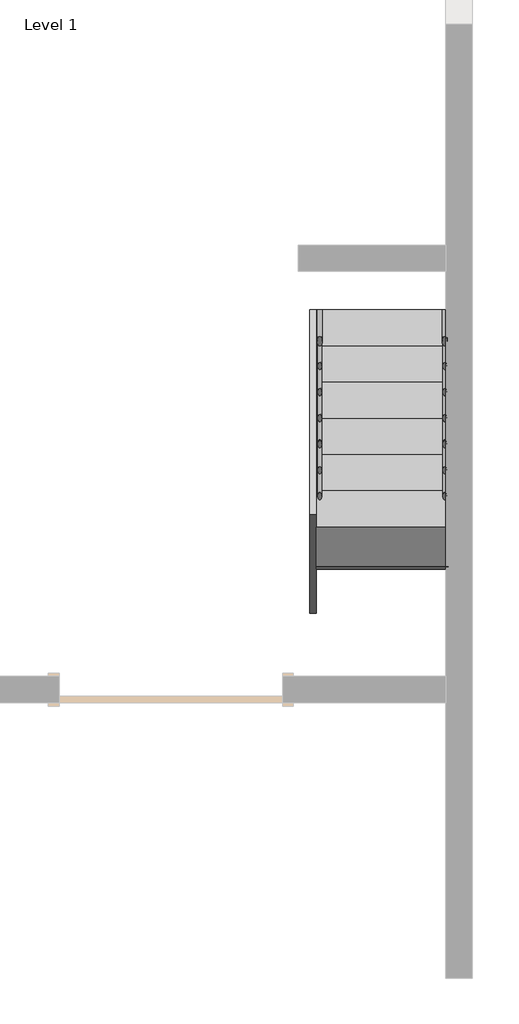
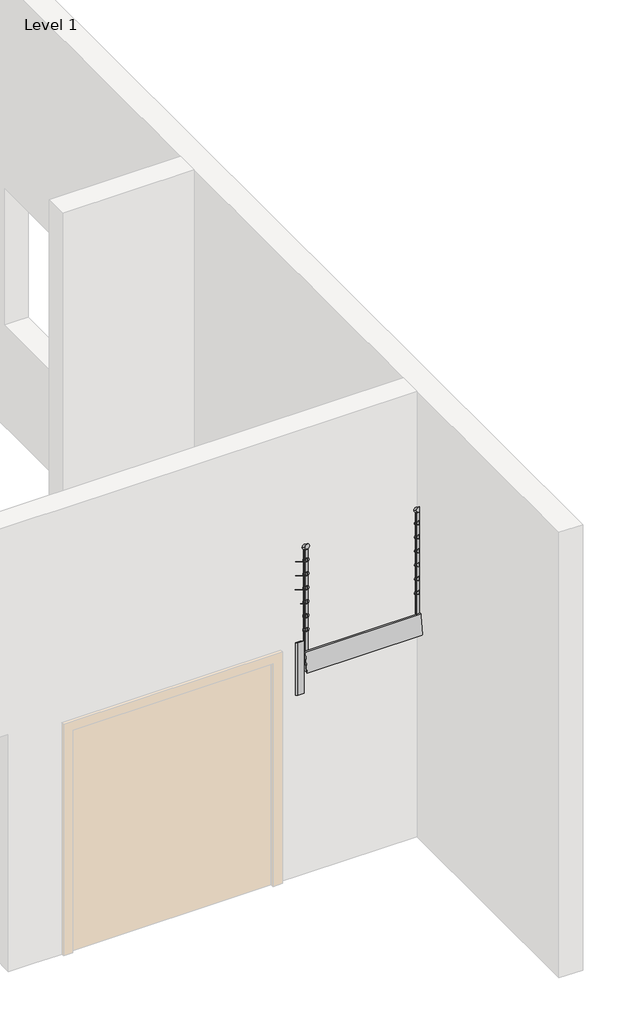
# One storey, part 2 of 2: 2 members, 2 railings, 1 stair flight.
"""IFC4 building model written with IfcOpenShell, lengths in millimetres."""

from ifc_helpers import new_model, si_unit, frame, origin, place, context, project, spatial, polyline, circle_curve, ellipse_curve, outline, extrude, transform, mapped, element, save
from ifc_brep_helpers import plane_surface, cylinder_surface, advanced_brep
from components import stair_flight_50mm_tread_25mm_nosing_13mm_riser_4d1d0ec9

model = new_model("IFC4")

# Units and contexts
model_context = context("Model", 3, world=origin())
ifc_project = project(units=[si_unit("LENGTHUNIT", "METRE", prefix="MILLI")], contexts=[model_context])

# Site, building, storey
site = spatial("IfcSite", under=ifc_project)
building = spatial("IfcBuilding", under=site)
storey = spatial("IfcBuildingStorey", under=building, Name="Level 1", Elevation=0.0)

# Members
placement = place(None, origin())
element("IfcMember", 1, ObjectType="Stringer - 50mm Width", at=placement, inside=storey, context=model_context, shape_type="SweptSolid", body=[
    extrude(outline(polyline([(358.5943271, 215.089535), (358.5943271, 0.0), (-49.6644057, 0.0), (-2666.4056729, 1654.8561374), (-2666.4056729, 2128.1330133), (358.5943271, 215.089535)])), frame((-692.5027035, 0.0, 0.0), z_axis=(1.0, 0.0, 0.0), x_axis=(0.0, 1.0, 0.0)), (0.0, 0.0, 1.0), 50.0),
])
element("IfcMember", 2, ObjectType="Stringer - 50mm Width", at=placement, inside=storey, context=model_context, shape_type="SweptSolid", body=[
    extrude(outline(polyline([(358.5943271, 215.089535), (358.5943271, 0.0), (-49.6644057, 0.0), (-2666.4056729, 1654.8561374), (-2666.4056729, 2128.1330133), (358.5943271, 215.089535)])), frame((-1742.5284847, 0.0, 0.0), z_axis=(1.0, 0.0, 0.0), x_axis=(0.0, 1.0, 0.0)), (0.0, 0.0, 1.0), 50.0),
])

# Railings
element("IfcRailing", 3, ObjectType="900mm Pipe", at=placement, inside=storey, context=model_context, shape_type="AdvancedBrep", body=[
    advanced_brep(
    [(-1687.1284847, 358.5943271, 1050.2491997), (-1647.1284847, 358.5943271, 1050.2491997), (-1687.1284847, -2666.4056729, 2963.2926779), (-1647.1284847, -2666.4056729, 2963.2926779)],
    [
        (0, 1, ellipse_curve(frame((-1667.1284847, 358.5943271, 1050.2491997), z_axis=(0.0, 1.0, 0.0), x_axis=(0.0, 0.0, -1.0)), 23.6638438, 20.0)),
        (1, 0, ellipse_curve(frame((-1667.1284847, 358.5943271, 1050.2491997), z_axis=(0.0, 1.0, 0.0), x_axis=(0.0, 0.0, -1.0)), 23.6638438, 20.0)),
        (2, 3, ellipse_curve(frame((-1667.1284847, -2666.4056729, 2963.2926779), z_axis=(0.0, -1.0, 0.0), x_axis=(0.0, 0.0, -1.0)), 23.6638438, 20.0)),
        (3, 2, ellipse_curve(frame((-1667.1284847, -2666.4056729, 2963.2926779), z_axis=(0.0, -1.0, 0.0), x_axis=(0.0, 0.0, -1.0)), 23.6638438, 20.0)),
        (0, 2),
        (3, 1),
    ],
    [
        plane_surface(frame((-1667.1284847, 358.5943271, 1073.9130435), z_axis=(0.0, 1.0, 0.0), x_axis=(0.0, 0.0, -1.0))),
        plane_surface(frame((-1667.1284847, -2666.4056729, 2986.9565217), z_axis=(0.0, -1.0, 0.0), x_axis=(0.0, 0.0, -1.0))),
        cylinder_surface(frame((-1667.1284847, 347.9044143, 1057.0096189), z_axis=(0.0, 0.8451712313980438, -0.5344956404098301), x_axis=(1.0, 0.0, 0.0)), 20.0),
    ],
    [
        (0, [[1, 2]]),
        (1, [[3, 4]]),
        (2, [[-1, 5, -4, 6]]),
        (2, [[-2, -6, -3, -5]]),
    ],
),
    advanced_brep(
    [(-1652.1284847, 358.5943271, 931.1651606), (-1682.1284847, 358.5943271, 931.1651606), (-1652.1284847, -2666.4056729, 2844.2086389), (-1682.1284847, -2666.4056729, 2844.2086389)],
    [
        (0, 1, ellipse_curve(frame((-1667.1284847, 358.5943271, 931.1651606), z_axis=(0.0, 1.0, 0.0), x_axis=(0.0, 0.0, -1.0)), 17.7478828, 15.0)),
        (1, 0, ellipse_curve(frame((-1667.1284847, 358.5943271, 931.1651606), z_axis=(0.0, 1.0, 0.0), x_axis=(0.0, 0.0, -1.0)), 17.7478828, 15.0)),
        (2, 3, ellipse_curve(frame((-1667.1284847, -2666.4056729, 2844.2086389), z_axis=(0.0, -1.0, 0.0), x_axis=(0.0, 0.0, -1.0)), 17.7478828, 15.0)),
        (3, 2, ellipse_curve(frame((-1667.1284847, -2666.4056729, 2844.2086389), z_axis=(0.0, -1.0, 0.0), x_axis=(0.0, 0.0, -1.0)), 17.7478828, 15.0)),
        (0, 2),
        (3, 1),
    ],
    [
        plane_surface(frame((-1667.1284847, 358.5943271, 948.9130435), z_axis=(0.0, 1.0, 0.0), x_axis=(0.0, 0.0, -1.0))),
        plane_surface(frame((-1667.1284847, -2666.4056729, 2861.9565217), z_axis=(0.0, -1.0, 0.0), x_axis=(0.0, 0.0, -1.0))),
        cylinder_surface(frame((-1667.1284847, 350.5768925, 936.235475), z_axis=(0.0, 0.8451712313980438, -0.5344956404098301), x_axis=(-1.0, 0.0, 0.0)), 15.0),
    ],
    [
        (0, [[1, 2]]),
        (1, [[3, 4]]),
        (2, [[-1, 5, -4, 6]]),
        (2, [[-2, -6, -3, -5]]),
    ],
),
    advanced_brep(
    [(-1652.1284847, 358.5943271, 806.1651606), (-1682.1284847, 358.5943271, 806.1651606), (-1652.1284847, -2666.4056729, 2719.2086389), (-1682.1284847, -2666.4056729, 2719.2086389)],
    [
        (0, 1, ellipse_curve(frame((-1667.1284847, 358.5943271, 806.1651606), z_axis=(0.0, 1.0, 0.0), x_axis=(0.0, 0.0, -1.0)), 17.7478828, 15.0)),
        (1, 0, ellipse_curve(frame((-1667.1284847, 358.5943271, 806.1651606), z_axis=(0.0, 1.0, 0.0), x_axis=(0.0, 0.0, -1.0)), 17.7478828, 15.0)),
        (2, 3, ellipse_curve(frame((-1667.1284847, -2666.4056729, 2719.2086389), z_axis=(0.0, -1.0, 0.0), x_axis=(0.0, 0.0, -1.0)), 17.7478828, 15.0)),
        (3, 2, ellipse_curve(frame((-1667.1284847, -2666.4056729, 2719.2086389), z_axis=(0.0, -1.0, 0.0), x_axis=(0.0, 0.0, -1.0)), 17.7478828, 15.0)),
        (0, 2),
        (3, 1),
    ],
    [
        plane_surface(frame((-1667.1284847, 358.5943271, 823.9130435), z_axis=(0.0, 1.0, 0.0), x_axis=(0.0, 0.0, -1.0))),
        plane_surface(frame((-1667.1284847, -2666.4056729, 2736.9565217), z_axis=(0.0, -1.0, 0.0), x_axis=(0.0, 0.0, -1.0))),
        cylinder_surface(frame((-1667.1284847, 350.5768925, 811.235475), z_axis=(0.0, 0.8451712313980438, -0.5344956404098301), x_axis=(-1.0, 0.0, 0.0)), 15.0),
    ],
    [
        (0, [[1, 2]]),
        (1, [[3, 4]]),
        (2, [[-1, 5, -4, 6]]),
        (2, [[-2, -6, -3, -5]]),
    ],
),
    advanced_brep(
    [(-1652.1284847, 358.5943271, 681.1651606), (-1682.1284847, 358.5943271, 681.1651606), (-1652.1284847, -2666.4056729, 2594.2086389), (-1682.1284847, -2666.4056729, 2594.2086389)],
    [
        (0, 1, ellipse_curve(frame((-1667.1284847, 358.5943271, 681.1651606), z_axis=(0.0, 1.0, 0.0), x_axis=(0.0, 0.0, -1.0)), 17.7478828, 15.0)),
        (1, 0, ellipse_curve(frame((-1667.1284847, 358.5943271, 681.1651606), z_axis=(0.0, 1.0, 0.0), x_axis=(0.0, 0.0, -1.0)), 17.7478828, 15.0)),
        (2, 3, ellipse_curve(frame((-1667.1284847, -2666.4056729, 2594.2086389), z_axis=(0.0, -1.0, 0.0), x_axis=(0.0, 0.0, -1.0)), 17.7478828, 15.0)),
        (3, 2, ellipse_curve(frame((-1667.1284847, -2666.4056729, 2594.2086389), z_axis=(0.0, -1.0, 0.0), x_axis=(0.0, 0.0, -1.0)), 17.7478828, 15.0)),
        (0, 2),
        (3, 1),
    ],
    [
        plane_surface(frame((-1667.1284847, 358.5943271, 698.9130435), z_axis=(0.0, 1.0, 0.0), x_axis=(0.0, 0.0, -1.0))),
        plane_surface(frame((-1667.1284847, -2666.4056729, 2611.9565217), z_axis=(0.0, -1.0, 0.0), x_axis=(0.0, 0.0, -1.0))),
        cylinder_surface(frame((-1667.1284847, 350.5768925, 686.235475), z_axis=(0.0, 0.8451712313980438, -0.5344956404098301), x_axis=(-1.0, 0.0, 0.0)), 15.0),
    ],
    [
        (0, [[1, 2]]),
        (1, [[3, 4]]),
        (2, [[-1, 5, -4, 6]]),
        (2, [[-2, -6, -3, -5]]),
    ],
),
    advanced_brep(
    [(-1652.1284847, 358.5943271, 556.1651606), (-1682.1284847, 358.5943271, 556.1651606), (-1652.1284847, -2666.4056729, 2469.2086389), (-1682.1284847, -2666.4056729, 2469.2086389)],
    [
        (0, 1, ellipse_curve(frame((-1667.1284847, 358.5943271, 556.1651606), z_axis=(0.0, 1.0, 0.0), x_axis=(0.0, 0.0, -1.0)), 17.7478828, 15.0)),
        (1, 0, ellipse_curve(frame((-1667.1284847, 358.5943271, 556.1651606), z_axis=(0.0, 1.0, 0.0), x_axis=(0.0, 0.0, -1.0)), 17.7478828, 15.0)),
        (2, 3, ellipse_curve(frame((-1667.1284847, -2666.4056729, 2469.2086389), z_axis=(0.0, -1.0, 0.0), x_axis=(0.0, 0.0, -1.0)), 17.7478828, 15.0)),
        (3, 2, ellipse_curve(frame((-1667.1284847, -2666.4056729, 2469.2086389), z_axis=(0.0, -1.0, 0.0), x_axis=(0.0, 0.0, -1.0)), 17.7478828, 15.0)),
        (0, 2),
        (3, 1),
    ],
    [
        plane_surface(frame((-1667.1284847, 358.5943271, 573.9130435), z_axis=(0.0, 1.0, 0.0), x_axis=(0.0, 0.0, -1.0))),
        plane_surface(frame((-1667.1284847, -2666.4056729, 2486.9565217), z_axis=(0.0, -1.0, 0.0), x_axis=(0.0, 0.0, -1.0))),
        cylinder_surface(frame((-1667.1284847, 350.5768925, 561.235475), z_axis=(0.0, 0.845171231398044, -0.53449564040983), x_axis=(-1.0, 0.0, 0.0)), 15.0),
    ],
    [
        (0, [[1, 2]]),
        (1, [[3, 4]]),
        (2, [[-1, 5, -4, 6]]),
        (2, [[-2, -6, -3, -5]]),
    ],
),
    advanced_brep(
    [(-1652.1284847, 358.5943271, 431.1651606), (-1682.1284847, 358.5943271, 431.1651606), (-1652.1284847, -2666.4056729, 2344.2086389), (-1682.1284847, -2666.4056729, 2344.2086389)],
    [
        (0, 1, ellipse_curve(frame((-1667.1284847, 358.5943271, 431.1651606), z_axis=(0.0, 1.0, 0.0), x_axis=(0.0, 0.0, -1.0)), 17.7478828, 15.0)),
        (1, 0, ellipse_curve(frame((-1667.1284847, 358.5943271, 431.1651606), z_axis=(0.0, 1.0, 0.0), x_axis=(0.0, 0.0, -1.0)), 17.7478828, 15.0)),
        (2, 3, ellipse_curve(frame((-1667.1284847, -2666.4056729, 2344.2086389), z_axis=(0.0, -1.0, 0.0), x_axis=(0.0, 0.0, -1.0)), 17.7478828, 15.0)),
        (3, 2, ellipse_curve(frame((-1667.1284847, -2666.4056729, 2344.2086389), z_axis=(0.0, -1.0, 0.0), x_axis=(0.0, 0.0, -1.0)), 17.7478828, 15.0)),
        (0, 2),
        (3, 1),
    ],
    [
        plane_surface(frame((-1667.1284847, 358.5943271, 448.9130435), z_axis=(0.0, 1.0, 0.0), x_axis=(0.0, 0.0, -1.0))),
        plane_surface(frame((-1667.1284847, -2666.4056729, 2361.9565217), z_axis=(0.0, -1.0, 0.0), x_axis=(0.0, 0.0, -1.0))),
        cylinder_surface(frame((-1667.1284847, 350.5768925, 436.235475), z_axis=(0.0, 0.8451712313980438, -0.5344956404098301), x_axis=(-1.0, 0.0, 0.0)), 15.0),
    ],
    [
        (0, [[1, 2]]),
        (1, [[3, 4]]),
        (2, [[-1, 5, -4, 6]]),
        (2, [[-2, -6, -3, -5]]),
    ],
),
    advanced_brep(
    [(-1652.1284847, 358.5943271, 306.1651606), (-1682.1284847, 358.5943271, 306.1651606), (-1652.1284847, -2666.4056729, 2219.2086389), (-1682.1284847, -2666.4056729, 2219.2086389)],
    [
        (0, 1, ellipse_curve(frame((-1667.1284847, 358.5943271, 306.1651606), z_axis=(0.0, 1.0, 0.0), x_axis=(0.0, 0.0, -1.0)), 17.7478828, 15.0)),
        (1, 0, ellipse_curve(frame((-1667.1284847, 358.5943271, 306.1651606), z_axis=(0.0, 1.0, 0.0), x_axis=(0.0, 0.0, -1.0)), 17.7478828, 15.0)),
        (2, 3, ellipse_curve(frame((-1667.1284847, -2666.4056729, 2219.2086389), z_axis=(0.0, -1.0, 0.0), x_axis=(0.0, 0.0, -1.0)), 17.7478828, 15.0)),
        (3, 2, ellipse_curve(frame((-1667.1284847, -2666.4056729, 2219.2086389), z_axis=(0.0, -1.0, 0.0), x_axis=(0.0, 0.0, -1.0)), 17.7478828, 15.0)),
        (0, 2),
        (3, 1),
    ],
    [
        plane_surface(frame((-1667.1284847, 358.5943271, 323.9130435), z_axis=(0.0, 1.0, 0.0), x_axis=(0.0, 0.0, -1.0))),
        plane_surface(frame((-1667.1284847, -2666.4056729, 2236.9565217), z_axis=(0.0, -1.0, 0.0), x_axis=(0.0, 0.0, -1.0))),
        cylinder_surface(frame((-1667.1284847, 350.5768925, 311.235475), z_axis=(0.0, 0.8451712313980438, -0.5344956404098301), x_axis=(-1.0, 0.0, 0.0)), 15.0),
    ],
    [
        (0, [[1, 2]]),
        (1, [[3, 4]]),
        (2, [[-1, 5, -4, 6]]),
        (2, [[-2, -6, -3, -5]]),
    ],
),
    advanced_brep(
    [(-1679.6284847, -2641.4056729, 2923.8185575), (-1679.6284847, -2641.4056729, 1913.0434783), (-1654.6284847, -2641.4056729, 1913.0434783), (-1654.6284847, -2641.4056729, 2923.8185575)],
    [
        (0, 1),
        (1, 2, circle_curve(frame((-1667.1284847, -2641.4056729, 1913.0434783), z_axis=(0.0, 0.0, 1.0), x_axis=(1.0, 0.0, 0.0)), 12.5)),
        (2, 3),
        (3, 0, ellipse_curve(frame((-1667.1284847, -2641.4056729, 2923.8185575), z_axis=(0.0, -0.5344956404098302, -0.8451712313980437), x_axis=(0.0, -0.8451712313980437, 0.53449564040983)), 14.7899024, 12.5)),
        (0, 3, ellipse_curve(frame((-1667.1284847, -2641.4056729, 2923.8185575), z_axis=(0.0, -0.5344956404098302, -0.8451712313980437), x_axis=(0.0, -0.8451712313980437, 0.53449564040983)), 14.7899024, 12.5)),
        (2, 1, circle_curve(frame((-1667.1284847, -2641.4056729, 1913.0434783), z_axis=(0.0, 0.0, 1.0), x_axis=(1.0, 0.0, 0.0)), 12.5)),
    ],
    [
        cylinder_surface(frame((-1667.1284847, -2641.4056729, 1813.0434783), z_axis=(0.0, 0.0, 1.0), x_axis=(1.0, 0.0, 0.0)), 12.5),
        plane_surface(frame((-1642.1284847, -2666.4056729, 2939.6288341), z_axis=(0.0, 0.5344956404098302, 0.8451712313980437), x_axis=(-1.0, 0.0, 0.0))),
        plane_surface(frame((-1642.1284847, -2616.4056729, 1913.0434783), z_axis=(0.0, 0.0, -1.0), x_axis=(-1.0, 0.0, 0.0))),
    ],
    [
        (0, [[1, 2, 3, 4]]),
        (0, [[-1, 5, -3, 6]]),
        (1, [[-4, -5]]),
        (2, [[-2, -6]]),
    ],
),
    advanced_brep(
    [(-1679.6284847, -1641.4056729, 2291.4074903), (-1679.6284847, -1641.4056729, 1391.3043478), (-1654.6284847, -1641.4056729, 1391.3043478), (-1654.6284847, -1641.4056729, 2291.4074903)],
    [
        (0, 1),
        (1, 2, circle_curve(frame((-1667.1284847, -1641.4056729, 1391.3043478), z_axis=(0.0, 0.0, 1.0), x_axis=(1.0, 0.0, 0.0)), 12.5)),
        (2, 3),
        (3, 0, ellipse_curve(frame((-1667.1284847, -1641.4056729, 2291.4074903), z_axis=(0.0, -0.5344956404098302, -0.8451712313980437), x_axis=(0.0, -0.8451712313980437, 0.53449564040983)), 14.7899024, 12.5)),
        (0, 3, ellipse_curve(frame((-1667.1284847, -1641.4056729, 2291.4074903), z_axis=(0.0, -0.5344956404098302, -0.8451712313980437), x_axis=(0.0, -0.8451712313980437, 0.53449564040983)), 14.7899024, 12.5)),
        (2, 1, circle_curve(frame((-1667.1284847, -1641.4056729, 1391.3043478), z_axis=(0.0, 0.0, 1.0), x_axis=(1.0, 0.0, 0.0)), 12.5)),
    ],
    [
        cylinder_surface(frame((-1667.1284847, -1641.4056729, 1291.3043478), z_axis=(0.0, 0.0, 1.0), x_axis=(1.0, 0.0, 0.0)), 12.5),
        plane_surface(frame((-1642.1284847, -1666.4056729, 2307.217767), z_axis=(0.0, 0.5344956404098302, 0.8451712313980437), x_axis=(-1.0, 0.0, 0.0))),
        plane_surface(frame((-1642.1284847, -1616.4056729, 1391.3043478), z_axis=(0.0, 0.0, -1.0), x_axis=(-1.0, 0.0, 0.0))),
    ],
    [
        (0, [[1, 2, 3, 4]]),
        (0, [[-1, 5, -3, 6]]),
        (1, [[-4, -5]]),
        (2, [[-2, -6]]),
    ],
),
    advanced_brep(
    [(-1679.6284847, -641.4056729, 1658.9964231), (-1679.6284847, -641.4056729, 695.6521739), (-1654.6284847, -641.4056729, 695.6521739), (-1654.6284847, -641.4056729, 1658.9964231)],
    [
        (0, 1),
        (1, 2, circle_curve(frame((-1667.1284847, -641.4056729, 695.6521739), z_axis=(0.0, 0.0, 1.0), x_axis=(1.0, 0.0, 0.0)), 12.5)),
        (2, 3),
        (3, 0, ellipse_curve(frame((-1667.1284847, -641.4056729, 1658.9964231), z_axis=(0.0, -0.5344956404098302, -0.8451712313980437), x_axis=(0.0, -0.8451712313980437, 0.53449564040983)), 14.7899024, 12.5)),
        (0, 3, ellipse_curve(frame((-1667.1284847, -641.4056729, 1658.9964231), z_axis=(0.0, -0.5344956404098302, -0.8451712313980437), x_axis=(0.0, -0.8451712313980437, 0.53449564040983)), 14.7899024, 12.5)),
        (2, 1, circle_curve(frame((-1667.1284847, -641.4056729, 695.6521739), z_axis=(0.0, 0.0, 1.0), x_axis=(1.0, 0.0, 0.0)), 12.5)),
    ],
    [
        cylinder_surface(frame((-1667.1284847, -641.4056729, 595.6521739), z_axis=(0.0, 0.0, 1.0), x_axis=(1.0, 0.0, 0.0)), 12.5),
        plane_surface(frame((-1642.1284847, -666.4056729, 1674.8066998), z_axis=(0.0, 0.5344956404098302, 0.8451712313980437), x_axis=(-1.0, 0.0, 0.0))),
        plane_surface(frame((-1642.1284847, -616.4056729, 695.6521739), z_axis=(0.0, 0.0, -1.0), x_axis=(-1.0, 0.0, 0.0))),
    ],
    [
        (0, [[1, 2, 3, 4]]),
        (0, [[-1, 5, -3, 6]]),
        (1, [[-4, -5]]),
        (2, [[-2, -6]]),
    ],
),
    advanced_brep(
    [(-1679.6284847, -2653.9056729, 2931.7236958), (-1679.6284847, -2653.9056729, 1913.0434783), (-1654.6284847, -2653.9056729, 1913.0434783), (-1654.6284847, -2653.9056729, 2931.7236958)],
    [
        (0, 1),
        (1, 2, circle_curve(frame((-1667.1284847, -2653.9056729, 1913.0434783), z_axis=(0.0, 0.0, 1.0), x_axis=(1.0, 0.0, 0.0)), 12.5)),
        (2, 3),
        (3, 0, ellipse_curve(frame((-1667.1284847, -2653.9056729, 2931.7236958), z_axis=(0.0, -0.5344956404098302, -0.8451712313980437), x_axis=(0.0, -0.8451712313980437, 0.53449564040983)), 14.7899024, 12.5)),
        (0, 3, ellipse_curve(frame((-1667.1284847, -2653.9056729, 2931.7236958), z_axis=(0.0, -0.5344956404098302, -0.8451712313980437), x_axis=(0.0, -0.8451712313980437, 0.53449564040983)), 14.7899024, 12.5)),
        (2, 1, circle_curve(frame((-1667.1284847, -2653.9056729, 1913.0434783), z_axis=(0.0, 0.0, 1.0), x_axis=(1.0, 0.0, 0.0)), 12.5)),
    ],
    [
        cylinder_surface(frame((-1667.1284847, -2653.9056729, 1813.0434783), z_axis=(0.0, 0.0, 1.0), x_axis=(1.0, 0.0, 0.0)), 12.5),
        plane_surface(frame((-1642.1284847, -2678.9056729, 2947.5339725), z_axis=(0.0, 0.5344956404098302, 0.8451712313980437), x_axis=(-1.0, 0.0, 0.0))),
        plane_surface(frame((-1642.1284847, -2628.9056729, 1913.0434783), z_axis=(0.0, 0.0, -1.0), x_axis=(-1.0, 0.0, 0.0))),
    ],
    [
        (0, [[1, 2, 3, 4]]),
        (0, [[-1, 5, -3, 6]]),
        (1, [[-4, -5]]),
        (2, [[-2, -6]]),
    ],
),
    advanced_brep(
    [(-1679.6284847, 346.0943271, 1034.4904942), (-1679.6284847, 346.0943271, 173.9130435), (-1654.6284847, 346.0943271, 173.9130435), (-1654.6284847, 346.0943271, 1034.4904942)],
    [
        (0, 1),
        (1, 2, circle_curve(frame((-1667.1284847, 346.0943271, 173.9130435), z_axis=(0.0, 0.0, 1.0), x_axis=(1.0, 0.0, 0.0)), 12.5)),
        (2, 3),
        (3, 0, ellipse_curve(frame((-1667.1284847, 346.0943271, 1034.4904942), z_axis=(0.0, -0.5344956404098302, -0.8451712313980437), x_axis=(0.0, -0.8451712313980437, 0.53449564040983)), 14.7899024, 12.5)),
        (0, 3, ellipse_curve(frame((-1667.1284847, 346.0943271, 1034.4904942), z_axis=(0.0, -0.5344956404098302, -0.8451712313980437), x_axis=(0.0, -0.8451712313980437, 0.53449564040983)), 14.7899024, 12.5)),
        (2, 1, circle_curve(frame((-1667.1284847, 346.0943271, 173.9130435), z_axis=(0.0, 0.0, 1.0), x_axis=(1.0, 0.0, 0.0)), 12.5)),
    ],
    [
        cylinder_surface(frame((-1667.1284847, 346.0943271, 73.9130435), z_axis=(0.0, 0.0, 1.0), x_axis=(1.0, 0.0, 0.0)), 12.5),
        plane_surface(frame((-1642.1284847, 321.0943271, 1050.3007709), z_axis=(0.0, 0.5344956404098302, 0.8451712313980437), x_axis=(-1.0, 0.0, 0.0))),
        plane_surface(frame((-1642.1284847, 371.0943271, 173.9130435), z_axis=(0.0, 0.0, -1.0), x_axis=(-1.0, 0.0, 0.0))),
    ],
    [
        (0, [[1, 2, 3, 4]]),
        (0, [[-1, 5, -3, 6]]),
        (1, [[-4, -5]]),
        (2, [[-2, -6]]),
    ],
),
])
element("IfcRailing", 4, ObjectType="900mm Pipe", at=placement, inside=storey, context=model_context, shape_type="AdvancedBrep", body=[
    advanced_brep(
    [(-737.9027035, 358.5943271, 1050.2491997), (-697.9027035, 358.5943271, 1050.2491997), (-737.9027035, -2666.4056729, 2963.2926779), (-697.9027035, -2666.4056729, 2963.2926779)],
    [
        (0, 1, ellipse_curve(frame((-717.9027035, 358.5943271, 1050.2491997), z_axis=(0.0, 1.0, 0.0), x_axis=(0.0, 0.0, -1.0)), 23.6638438, 20.0)),
        (1, 0, ellipse_curve(frame((-717.9027035, 358.5943271, 1050.2491997), z_axis=(0.0, 1.0, 0.0), x_axis=(0.0, 0.0, -1.0)), 23.6638438, 20.0)),
        (2, 3, ellipse_curve(frame((-717.9027035, -2666.4056729, 2963.2926779), z_axis=(0.0, -1.0, 0.0), x_axis=(0.0, 0.0, -1.0)), 23.6638438, 20.0)),
        (3, 2, ellipse_curve(frame((-717.9027035, -2666.4056729, 2963.2926779), z_axis=(0.0, -1.0, 0.0), x_axis=(0.0, 0.0, -1.0)), 23.6638438, 20.0)),
        (0, 2),
        (3, 1),
    ],
    [
        plane_surface(frame((-717.9027035, 358.5943271, 1073.9130435), z_axis=(0.0, 1.0, 0.0), x_axis=(0.0, 0.0, -1.0))),
        plane_surface(frame((-717.9027035, -2666.4056729, 2986.9565217), z_axis=(0.0, -1.0, 0.0), x_axis=(0.0, 0.0, -1.0))),
        cylinder_surface(frame((-717.9027035, 347.9044143, 1057.0096189), z_axis=(0.0, 0.8451712313980438, -0.5344956404098301), x_axis=(1.0, 0.0, 0.0)), 20.0),
    ],
    [
        (0, [[1, 2]]),
        (1, [[3, 4]]),
        (2, [[-1, 5, -4, 6]]),
        (2, [[-2, -6, -3, -5]]),
    ],
),
    advanced_brep(
    [(-732.9027035, 358.5943271, 931.1651606), (-702.9027035, 358.5943271, 931.1651606), (-732.9027035, -2666.4056729, 2844.2086389), (-702.9027035, -2666.4056729, 2844.2086389)],
    [
        (0, 1, ellipse_curve(frame((-717.9027035, 358.5943271, 931.1651606), z_axis=(0.0, 1.0, 0.0), x_axis=(0.0, 0.0, -1.0)), 17.7478828, 15.0)),
        (1, 0, ellipse_curve(frame((-717.9027035, 358.5943271, 931.1651606), z_axis=(0.0, 1.0, 0.0), x_axis=(0.0, 0.0, -1.0)), 17.7478828, 15.0)),
        (2, 3, ellipse_curve(frame((-717.9027035, -2666.4056729, 2844.2086389), z_axis=(0.0, -1.0, 0.0), x_axis=(0.0, 0.0, -1.0)), 17.7478828, 15.0)),
        (3, 2, ellipse_curve(frame((-717.9027035, -2666.4056729, 2844.2086389), z_axis=(0.0, -1.0, 0.0), x_axis=(0.0, 0.0, -1.0)), 17.7478828, 15.0)),
        (0, 2),
        (3, 1),
    ],
    [
        plane_surface(frame((-717.9027035, 358.5943271, 948.9130435), z_axis=(0.0, 1.0, 0.0), x_axis=(0.0, 0.0, -1.0))),
        plane_surface(frame((-717.9027035, -2666.4056729, 2861.9565217), z_axis=(0.0, -1.0, 0.0), x_axis=(0.0, 0.0, -1.0))),
        cylinder_surface(frame((-717.9027035, 350.5768925, 936.235475), z_axis=(0.0, 0.8451712313980438, -0.5344956404098301), x_axis=(1.0, 0.0, 0.0)), 15.0),
    ],
    [
        (0, [[1, 2]]),
        (1, [[3, 4]]),
        (2, [[-1, 5, -4, 6]]),
        (2, [[-2, -6, -3, -5]]),
    ],
),
    advanced_brep(
    [(-732.9027035, 358.5943271, 806.1651606), (-702.9027035, 358.5943271, 806.1651606), (-732.9027035, -2666.4056729, 2719.2086389), (-702.9027035, -2666.4056729, 2719.2086389)],
    [
        (0, 1, ellipse_curve(frame((-717.9027035, 358.5943271, 806.1651606), z_axis=(0.0, 1.0, 0.0), x_axis=(0.0, 0.0, -1.0)), 17.7478828, 15.0)),
        (1, 0, ellipse_curve(frame((-717.9027035, 358.5943271, 806.1651606), z_axis=(0.0, 1.0, 0.0), x_axis=(0.0, 0.0, -1.0)), 17.7478828, 15.0)),
        (2, 3, ellipse_curve(frame((-717.9027035, -2666.4056729, 2719.2086389), z_axis=(0.0, -1.0, 0.0), x_axis=(0.0, 0.0, -1.0)), 17.7478828, 15.0)),
        (3, 2, ellipse_curve(frame((-717.9027035, -2666.4056729, 2719.2086389), z_axis=(0.0, -1.0, 0.0), x_axis=(0.0, 0.0, -1.0)), 17.7478828, 15.0)),
        (0, 2),
        (3, 1),
    ],
    [
        plane_surface(frame((-717.9027035, 358.5943271, 823.9130435), z_axis=(0.0, 1.0, 0.0), x_axis=(0.0, 0.0, -1.0))),
        plane_surface(frame((-717.9027035, -2666.4056729, 2736.9565217), z_axis=(0.0, -1.0, 0.0), x_axis=(0.0, 0.0, -1.0))),
        cylinder_surface(frame((-717.9027035, 350.5768925, 811.235475), z_axis=(0.0, 0.8451712313980438, -0.5344956404098301), x_axis=(1.0, 0.0, 0.0)), 15.0),
    ],
    [
        (0, [[1, 2]]),
        (1, [[3, 4]]),
        (2, [[-1, 5, -4, 6]]),
        (2, [[-2, -6, -3, -5]]),
    ],
),
    advanced_brep(
    [(-732.9027035, 358.5943271, 681.1651606), (-702.9027035, 358.5943271, 681.1651606), (-732.9027035, -2666.4056729, 2594.2086389), (-702.9027035, -2666.4056729, 2594.2086389)],
    [
        (0, 1, ellipse_curve(frame((-717.9027035, 358.5943271, 681.1651606), z_axis=(0.0, 1.0, 0.0), x_axis=(0.0, 0.0, -1.0)), 17.7478828, 15.0)),
        (1, 0, ellipse_curve(frame((-717.9027035, 358.5943271, 681.1651606), z_axis=(0.0, 1.0, 0.0), x_axis=(0.0, 0.0, -1.0)), 17.7478828, 15.0)),
        (2, 3, ellipse_curve(frame((-717.9027035, -2666.4056729, 2594.2086389), z_axis=(0.0, -1.0, 0.0), x_axis=(0.0, 0.0, -1.0)), 17.7478828, 15.0)),
        (3, 2, ellipse_curve(frame((-717.9027035, -2666.4056729, 2594.2086389), z_axis=(0.0, -1.0, 0.0), x_axis=(0.0, 0.0, -1.0)), 17.7478828, 15.0)),
        (0, 2),
        (3, 1),
    ],
    [
        plane_surface(frame((-717.9027035, 358.5943271, 698.9130435), z_axis=(0.0, 1.0, 0.0), x_axis=(0.0, 0.0, -1.0))),
        plane_surface(frame((-717.9027035, -2666.4056729, 2611.9565217), z_axis=(0.0, -1.0, 0.0), x_axis=(0.0, 0.0, -1.0))),
        cylinder_surface(frame((-717.9027035, 350.5768925, 686.235475), z_axis=(0.0, 0.8451712313980438, -0.53449564040983), x_axis=(1.0, 0.0, 0.0)), 15.0),
    ],
    [
        (0, [[1, 2]]),
        (1, [[3, 4]]),
        (2, [[-1, 5, -4, 6]]),
        (2, [[-2, -6, -3, -5]]),
    ],
),
    advanced_brep(
    [(-732.9027035, 358.5943271, 556.1651606), (-702.9027035, 358.5943271, 556.1651606), (-732.9027035, -2666.4056729, 2469.2086389), (-702.9027035, -2666.4056729, 2469.2086389)],
    [
        (0, 1, ellipse_curve(frame((-717.9027035, 358.5943271, 556.1651606), z_axis=(0.0, 1.0, 0.0), x_axis=(0.0, 0.0, -1.0)), 17.7478828, 15.0)),
        (1, 0, ellipse_curve(frame((-717.9027035, 358.5943271, 556.1651606), z_axis=(0.0, 1.0, 0.0), x_axis=(0.0, 0.0, -1.0)), 17.7478828, 15.0)),
        (2, 3, ellipse_curve(frame((-717.9027035, -2666.4056729, 2469.2086389), z_axis=(0.0, -1.0, 0.0), x_axis=(0.0, 0.0, -1.0)), 17.7478828, 15.0)),
        (3, 2, ellipse_curve(frame((-717.9027035, -2666.4056729, 2469.2086389), z_axis=(0.0, -1.0, 0.0), x_axis=(0.0, 0.0, -1.0)), 17.7478828, 15.0)),
        (0, 2),
        (3, 1),
    ],
    [
        plane_surface(frame((-717.9027035, 358.5943271, 573.9130435), z_axis=(0.0, 1.0, 0.0), x_axis=(0.0, 0.0, -1.0))),
        plane_surface(frame((-717.9027035, -2666.4056729, 2486.9565217), z_axis=(0.0, -1.0, 0.0), x_axis=(0.0, 0.0, -1.0))),
        cylinder_surface(frame((-717.9027035, 350.5768925, 561.235475), z_axis=(0.0, 0.8451712313980438, -0.5344956404098301), x_axis=(1.0, 0.0, 0.0)), 15.0),
    ],
    [
        (0, [[1, 2]]),
        (1, [[3, 4]]),
        (2, [[-1, 5, -4, 6]]),
        (2, [[-2, -6, -3, -5]]),
    ],
),
    advanced_brep(
    [(-732.9027035, 358.5943271, 431.1651606), (-702.9027035, 358.5943271, 431.1651606), (-732.9027035, -2666.4056729, 2344.2086389), (-702.9027035, -2666.4056729, 2344.2086389)],
    [
        (0, 1, ellipse_curve(frame((-717.9027035, 358.5943271, 431.1651606), z_axis=(0.0, 1.0, 0.0), x_axis=(0.0, 0.0, -1.0)), 17.7478828, 15.0)),
        (1, 0, ellipse_curve(frame((-717.9027035, 358.5943271, 431.1651606), z_axis=(0.0, 1.0, 0.0), x_axis=(0.0, 0.0, -1.0)), 17.7478828, 15.0)),
        (2, 3, ellipse_curve(frame((-717.9027035, -2666.4056729, 2344.2086389), z_axis=(0.0, -1.0, 0.0), x_axis=(0.0, 0.0, -1.0)), 17.7478828, 15.0)),
        (3, 2, ellipse_curve(frame((-717.9027035, -2666.4056729, 2344.2086389), z_axis=(0.0, -1.0, 0.0), x_axis=(0.0, 0.0, -1.0)), 17.7478828, 15.0)),
        (0, 2),
        (3, 1),
    ],
    [
        plane_surface(frame((-717.9027035, 358.5943271, 448.9130435), z_axis=(0.0, 1.0, 0.0), x_axis=(0.0, 0.0, -1.0))),
        plane_surface(frame((-717.9027035, -2666.4056729, 2361.9565217), z_axis=(0.0, -1.0, 0.0), x_axis=(0.0, 0.0, -1.0))),
        cylinder_surface(frame((-717.9027035, 350.5768925, 436.235475), z_axis=(0.0, 0.8451712313980438, -0.5344956404098301), x_axis=(1.0, 0.0, 0.0)), 15.0),
    ],
    [
        (0, [[1, 2]]),
        (1, [[3, 4]]),
        (2, [[-1, 5, -4, 6]]),
        (2, [[-2, -6, -3, -5]]),
    ],
),
    advanced_brep(
    [(-732.9027035, 358.5943271, 306.1651606), (-702.9027035, 358.5943271, 306.1651606), (-732.9027035, -2666.4056729, 2219.2086389), (-702.9027035, -2666.4056729, 2219.2086389)],
    [
        (0, 1, ellipse_curve(frame((-717.9027035, 358.5943271, 306.1651606), z_axis=(0.0, 1.0, 0.0), x_axis=(0.0, 0.0, -1.0)), 17.7478828, 15.0)),
        (1, 0, ellipse_curve(frame((-717.9027035, 358.5943271, 306.1651606), z_axis=(0.0, 1.0, 0.0), x_axis=(0.0, 0.0, -1.0)), 17.7478828, 15.0)),
        (2, 3, ellipse_curve(frame((-717.9027035, -2666.4056729, 2219.2086389), z_axis=(0.0, -1.0, 0.0), x_axis=(0.0, 0.0, -1.0)), 17.7478828, 15.0)),
        (3, 2, ellipse_curve(frame((-717.9027035, -2666.4056729, 2219.2086389), z_axis=(0.0, -1.0, 0.0), x_axis=(0.0, 0.0, -1.0)), 17.7478828, 15.0)),
        (0, 2),
        (3, 1),
    ],
    [
        plane_surface(frame((-717.9027035, 358.5943271, 323.9130435), z_axis=(0.0, 1.0, 0.0), x_axis=(0.0, 0.0, -1.0))),
        plane_surface(frame((-717.9027035, -2666.4056729, 2236.9565217), z_axis=(0.0, -1.0, 0.0), x_axis=(0.0, 0.0, -1.0))),
        cylinder_surface(frame((-717.9027035, 350.5768925, 311.235475), z_axis=(0.0, 0.8451712313980438, -0.5344956404098301), x_axis=(1.0, 0.0, 0.0)), 15.0),
    ],
    [
        (0, [[1, 2]]),
        (1, [[3, 4]]),
        (2, [[-1, 5, -4, 6]]),
        (2, [[-2, -6, -3, -5]]),
    ],
),
    advanced_brep(
    [(-705.4027035, -2641.4056729, 2923.8185575), (-730.4027035, -2641.4056729, 2923.8185575), (-730.4027035, -2641.4056729, 1913.0434783), (-705.4027035, -2641.4056729, 1913.0434783)],
    [
        (0, 1, ellipse_curve(frame((-717.9027035, -2641.4056729, 2923.8185575), z_axis=(0.0, -0.5344956404098302, -0.8451712313980437), x_axis=(0.0, -0.8451712313980437, 0.53449564040983)), 14.7899024, 12.5)),
        (1, 2),
        (2, 3, circle_curve(frame((-717.9027035, -2641.4056729, 1913.0434783), z_axis=(0.0, 0.0, 1.0), x_axis=(-1.0, 0.0, 0.0)), 12.5)),
        (3, 0),
        (3, 2, circle_curve(frame((-717.9027035, -2641.4056729, 1913.0434783), z_axis=(0.0, 0.0, 1.0), x_axis=(-1.0, 0.0, 0.0)), 12.5)),
        (1, 0, ellipse_curve(frame((-717.9027035, -2641.4056729, 2923.8185575), z_axis=(0.0, -0.5344956404098302, -0.8451712313980437), x_axis=(0.0, -0.8451712313980437, 0.53449564040983)), 14.7899024, 12.5)),
    ],
    [
        cylinder_surface(frame((-717.9027035, -2641.4056729, 1813.0434783), z_axis=(0.0, 0.0, 1.0), x_axis=(-1.0, 0.0, 0.0)), 12.5),
        plane_surface(frame((-742.9027035, -2666.4056729, 2939.6288341), z_axis=(0.0, 0.5344956404098302, 0.8451712313980437), x_axis=(1.0, 0.0, 0.0))),
        plane_surface(frame((-742.9027035, -2616.4056729, 1913.0434783), z_axis=(0.0, 0.0, -1.0), x_axis=(1.0, 0.0, 0.0))),
    ],
    [
        (0, [[1, 2, 3, 4]]),
        (0, [[5, -2, 6, -4]]),
        (1, [[-6, -1]]),
        (2, [[-5, -3]]),
    ],
),
    advanced_brep(
    [(-705.4027035, -1641.4056729, 2291.4074903), (-730.4027035, -1641.4056729, 2291.4074903), (-730.4027035, -1641.4056729, 1391.3043478), (-705.4027035, -1641.4056729, 1391.3043478)],
    [
        (0, 1, ellipse_curve(frame((-717.9027035, -1641.4056729, 2291.4074903), z_axis=(0.0, -0.5344956404098302, -0.8451712313980437), x_axis=(0.0, -0.8451712313980437, 0.53449564040983)), 14.7899024, 12.5)),
        (1, 2),
        (2, 3, circle_curve(frame((-717.9027035, -1641.4056729, 1391.3043478), z_axis=(0.0, 0.0, 1.0), x_axis=(-1.0, 0.0, 0.0)), 12.5)),
        (3, 0),
        (3, 2, circle_curve(frame((-717.9027035, -1641.4056729, 1391.3043478), z_axis=(0.0, 0.0, 1.0), x_axis=(-1.0, 0.0, 0.0)), 12.5)),
        (1, 0, ellipse_curve(frame((-717.9027035, -1641.4056729, 2291.4074903), z_axis=(0.0, -0.5344956404098302, -0.8451712313980437), x_axis=(0.0, -0.8451712313980437, 0.53449564040983)), 14.7899024, 12.5)),
    ],
    [
        cylinder_surface(frame((-717.9027035, -1641.4056729, 1291.3043478), z_axis=(0.0, 0.0, 1.0), x_axis=(-1.0, 0.0, 0.0)), 12.5),
        plane_surface(frame((-742.9027035, -1666.4056729, 2307.217767), z_axis=(0.0, 0.5344956404098302, 0.8451712313980437), x_axis=(1.0, 0.0, 0.0))),
        plane_surface(frame((-742.9027035, -1616.4056729, 1391.3043478), z_axis=(0.0, 0.0, -1.0), x_axis=(1.0, 0.0, 0.0))),
    ],
    [
        (0, [[1, 2, 3, 4]]),
        (0, [[5, -2, 6, -4]]),
        (1, [[-6, -1]]),
        (2, [[-5, -3]]),
    ],
),
    advanced_brep(
    [(-705.4027035, -641.4056729, 1658.9964231), (-730.4027035, -641.4056729, 1658.9964231), (-730.4027035, -641.4056729, 695.6521739), (-705.4027035, -641.4056729, 695.6521739)],
    [
        (0, 1, ellipse_curve(frame((-717.9027035, -641.4056729, 1658.9964231), z_axis=(0.0, -0.5344956404098302, -0.8451712313980437), x_axis=(0.0, -0.8451712313980437, 0.53449564040983)), 14.7899024, 12.5)),
        (1, 2),
        (2, 3, circle_curve(frame((-717.9027035, -641.4056729, 695.6521739), z_axis=(0.0, 0.0, 1.0), x_axis=(-1.0, 0.0, 0.0)), 12.5)),
        (3, 0),
        (3, 2, circle_curve(frame((-717.9027035, -641.4056729, 695.6521739), z_axis=(0.0, 0.0, 1.0), x_axis=(-1.0, 0.0, 0.0)), 12.5)),
        (1, 0, ellipse_curve(frame((-717.9027035, -641.4056729, 1658.9964231), z_axis=(0.0, -0.5344956404098302, -0.8451712313980437), x_axis=(0.0, -0.8451712313980437, 0.53449564040983)), 14.7899024, 12.5)),
    ],
    [
        cylinder_surface(frame((-717.9027035, -641.4056729, 595.6521739), z_axis=(0.0, 0.0, 1.0), x_axis=(-1.0, 0.0, 0.0)), 12.5),
        plane_surface(frame((-742.9027035, -666.4056729, 1674.8066998), z_axis=(0.0, 0.5344956404098302, 0.8451712313980437), x_axis=(1.0, 0.0, 0.0))),
        plane_surface(frame((-742.9027035, -616.4056729, 695.6521739), z_axis=(0.0, 0.0, -1.0), x_axis=(1.0, 0.0, 0.0))),
    ],
    [
        (0, [[1, 2, 3, 4]]),
        (0, [[5, -2, 6, -4]]),
        (1, [[-6, -1]]),
        (2, [[-5, -3]]),
    ],
),
    advanced_brep(
    [(-705.4027035, -2653.9056729, 2931.7236958), (-730.4027035, -2653.9056729, 2931.7236958), (-730.4027035, -2653.9056729, 1913.0434783), (-705.4027035, -2653.9056729, 1913.0434783)],
    [
        (0, 1, ellipse_curve(frame((-717.9027035, -2653.9056729, 2931.7236958), z_axis=(0.0, -0.5344956404098302, -0.8451712313980437), x_axis=(0.0, -0.8451712313980437, 0.53449564040983)), 14.7899024, 12.5)),
        (1, 2),
        (2, 3, circle_curve(frame((-717.9027035, -2653.9056729, 1913.0434783), z_axis=(0.0, 0.0, 1.0), x_axis=(-1.0, 0.0, 0.0)), 12.5)),
        (3, 0),
        (3, 2, circle_curve(frame((-717.9027035, -2653.9056729, 1913.0434783), z_axis=(0.0, 0.0, 1.0), x_axis=(-1.0, 0.0, 0.0)), 12.5)),
        (1, 0, ellipse_curve(frame((-717.9027035, -2653.9056729, 2931.7236958), z_axis=(0.0, -0.5344956404098302, -0.8451712313980437), x_axis=(0.0, -0.8451712313980437, 0.53449564040983)), 14.7899024, 12.5)),
    ],
    [
        cylinder_surface(frame((-717.9027035, -2653.9056729, 1813.0434783), z_axis=(0.0, 0.0, 1.0), x_axis=(-1.0, 0.0, 0.0)), 12.5),
        plane_surface(frame((-742.9027035, -2678.9056729, 2947.5339725), z_axis=(0.0, 0.5344956404098302, 0.8451712313980437), x_axis=(1.0, 0.0, 0.0))),
        plane_surface(frame((-742.9027035, -2628.9056729, 1913.0434783), z_axis=(0.0, 0.0, -1.0), x_axis=(1.0, 0.0, 0.0))),
    ],
    [
        (0, [[1, 2, 3, 4]]),
        (0, [[5, -2, 6, -4]]),
        (1, [[-6, -1]]),
        (2, [[-5, -3]]),
    ],
),
    advanced_brep(
    [(-705.4027035, 346.0943271, 1034.4904942), (-730.4027035, 346.0943271, 1034.4904942), (-730.4027035, 346.0943271, 173.9130435), (-705.4027035, 346.0943271, 173.9130435)],
    [
        (0, 1, ellipse_curve(frame((-717.9027035, 346.0943271, 1034.4904942), z_axis=(0.0, -0.5344956404098302, -0.8451712313980437), x_axis=(0.0, -0.8451712313980437, 0.53449564040983)), 14.7899024, 12.5)),
        (1, 2),
        (2, 3, circle_curve(frame((-717.9027035, 346.0943271, 173.9130435), z_axis=(0.0, 0.0, 1.0), x_axis=(-1.0, 0.0, 0.0)), 12.5)),
        (3, 0),
        (3, 2, circle_curve(frame((-717.9027035, 346.0943271, 173.9130435), z_axis=(0.0, 0.0, 1.0), x_axis=(-1.0, 0.0, 0.0)), 12.5)),
        (1, 0, ellipse_curve(frame((-717.9027035, 346.0943271, 1034.4904942), z_axis=(0.0, -0.5344956404098302, -0.8451712313980437), x_axis=(0.0, -0.8451712313980437, 0.53449564040983)), 14.7899024, 12.5)),
    ],
    [
        cylinder_surface(frame((-717.9027035, 346.0943271, 73.9130435), z_axis=(0.0, 0.0, 1.0), x_axis=(-1.0, 0.0, 0.0)), 12.5),
        plane_surface(frame((-742.9027035, 321.0943271, 1050.3007709), z_axis=(0.0, 0.5344956404098302, 0.8451712313980437), x_axis=(1.0, 0.0, 0.0))),
        plane_surface(frame((-742.9027035, 371.0943271, 173.9130435), z_axis=(0.0, 0.0, -1.0), x_axis=(1.0, 0.0, 0.0))),
    ],
    [
        (0, [[1, 2, 3, 4]]),
        (0, [[5, -2, 6, -4]]),
        (1, [[-6, -1]]),
        (2, [[-5, -3]]),
    ],
),
])

# Stair flight
stair_flight_50mm_tread_25mm_nosing_13mm_riser_shape = stair_flight_50mm_tread_25mm_nosing_13mm_riser_4d1d0ec9(model_context)
element("IfcStairFlight", 5, ObjectType="50mm Tread 25mm Nosing 13mm Riser", at=placement, inside=storey, context=model_context, shape_type="MappedRepresentation", body=[
    mapped(stair_flight_50mm_tread_25mm_nosing_13mm_riser_shape, transform((0.0, 0.0, 0.0), x_axis=(1.0, 0.0, 0.0), y_axis=(0.0, 1.0, 0.0), z_axis=(0.0, 0.0, 1.0))),
])

save(model, "model.ifc")

# Revit data of these elements
# Type "900mm Pipe"
#   built-in parameter 1008612 = 0.019685 (stored number, unit not read)
#   built-in parameter 1008611 = 0.0984252 (stored number, unit not read)
#   built-in parameter 1008609 = 6.56168 (stored number, unit not read)
#   built-in parameter 1008604 = 0.19685 (stored number, unit not read)
#   built-in parameter 1008603 = 0.164042 (stored number, unit not read)
#   Railing Height = 900 mm
#   built-in parameter 1008630 = 2
#   built-in parameter 1008610 = 2
#   built-in parameter 1008605 = 1
#   built-in parameter 1008618 = M_Baluster - Round : 25mm
# Elements 1, 2 (IfcMember, "Stringer - 50mm Width")
#   Phase Created = New Construction
# Elements 3, 4 (IfcRailing, "900mm Pipe")
#   Phase Created = New Construction
# Element 5 (IfcStairFlight, "50mm Tread 25mm Nosing 13mm Riser")
#   Phase Created = New Construction
